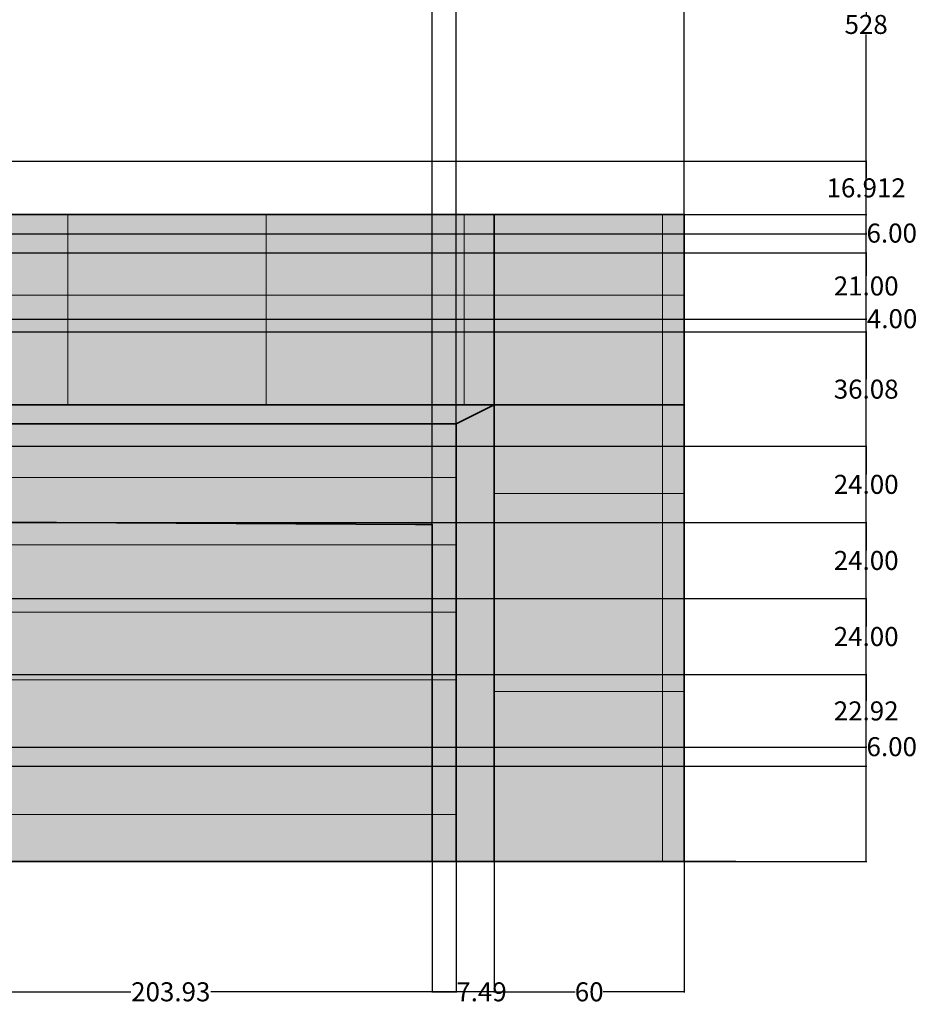
# Model space of a CAD drawing. Units: inches. Extents: x 148 to 1080, y 89 to 707.
# Tile 9 of 12: x 797 to 1080, y 89 to 399. Entities that reach past the tile are written whole.
import ezdxf

# ---------------------------------------------------------------- set-up
doc = ezdxf.new("R2010")
doc.units = ezdxf.units.IN
doc.header["$MEASUREMENT"] = 0
for name, color, linetype, lineweight in [('A-ANNO-DIMS', 2, 'Continuous', 18), ('A-ELEV', 7, 'Continuous', 35), ('A-ELEV-PATT', 8, 'Continuous', 13)]:
    doc.layers.add(name, color=color, linetype=linetype, lineweight=lineweight)
doc.styles.get("Standard").update_dxf_attribs({"font": 'arial.ttf'})
doc.dimstyles.get("Standard").update_dxf_attribs({"dimtxt": 6, "dimasz": 0.18, "dimexe": 0.18, "dimexo": 0.0625, "dimgap": 0.09, "dimtad": 0, "dimtih": 1, "dimtoh": 1, "dimdec": 0, "dimzin": 0, "dimdsep": 46, "dimlunit": 3, "dimtxsty": 'Standard', "dimcen": 0.09, "dimadec": 0, "dimazin": 0, "dimtfac": 1, "dimtdec": 0, "dimtofl": 0, "dimtmove": 0, "dimatfit": 3, "dimfxl": 1, "dimtolj": 1, "dimtzin": 0, "dimarcsym": 0})

# ---------------------------------------------------------------- blocks, each defined once
blk = doc.blocks.new('*D1')
at = {"layer": 'A-ANNO-DIMS', "color": 0, "lineweight": -2, "transparency": 16777216}
for p, q in [((215.02, 662.01), (215.02, 703.28)), ((215.2, 703.1), (604.32, 703.1)), ((1006.77, 703.1), (617.65, 703.1)), ((1006.95, 338.01), (1006.95, 703.28))]:
    blk.add_line(p, q, dxfattribs=at)
at = {"layer": 'A-ANNO-DIMS', "color": 0, "transparency": 16777216}
for points in [[(215.2, 703.13), (215.2, 703.07), (215.02, 703.1)], [(1006.77, 703.13), (1006.77, 703.07), (1006.95, 703.1)]]:
    blk.add_solid(points, dxfattribs=at)
at = {"layer": 'Defpoints', "color": 0, "transparency": 16777216}
for p in [(1006.95, 703.1), (215.02, 661.95), (1006.95, 337.95)]:
    blk.add_point(p, dxfattribs=at)
at = {"layer": 'A-ANNO-DIMS', "color": 0, "transparency": 16777216, "insert": (610.98, 703.1), "char_height": 6, "attachment_point": 5}
blk.add_mtext('\\A1;792', dxfattribs=at)
blk = doc.blocks.new('*D6')
at = {"layer": 'A-ANNO-DIMS', "color": 0, "lineweight": -2, "transparency": 16777216}
for p, q in [((743.02, 133.88), (743.02, 92.62)), ((946.95, 133.88), (946.95, 92.62)), ((743.2, 92.8), (832.39, 92.8)), ((946.77, 92.8), (857.58, 92.8))]:
    blk.add_line(p, q, dxfattribs=at)
at = {"layer": 'A-ANNO-DIMS', "color": 0, "transparency": 16777216}
for points in [[(743.2, 92.83), (743.2, 92.77), (743.02, 92.8)], [(946.77, 92.83), (946.77, 92.77), (946.95, 92.8)]]:
    blk.add_solid(points, dxfattribs=at)
at = {"layer": 'Defpoints', "color": 0, "transparency": 16777216}
for p in [(743.02, 133.95), (946.95, 133.95), (946.95, 92.8)]:
    blk.add_point(p, dxfattribs=at)
at = {"layer": 'A-ANNO-DIMS', "color": 0, "transparency": 16777216, "insert": (844.98, 92.8), "char_height": 6, "attachment_point": 5}
blk.add_mtext('\\A1;203.93', dxfattribs=at)
blk = doc.blocks.new('*D7')
at = {"layer": 'A-ANNO-DIMS', "color": 0, "lineweight": -2, "transparency": 16777216}
for p, q in [((946.95, 133.88), (946.95, 92.62)), ((1006.95, 133.88), (1006.95, 92.62)), ((947.13, 92.8), (972.56, 92.8)), ((1006.77, 92.8), (981.34, 92.8))]:
    blk.add_line(p, q, dxfattribs=at)
at = {"layer": 'A-ANNO-DIMS', "color": 0, "transparency": 16777216}
for points in [[(947.13, 92.83), (947.13, 92.77), (946.95, 92.8)], [(1006.77, 92.83), (1006.77, 92.77), (1006.95, 92.8)]]:
    blk.add_solid(points, dxfattribs=at)
at = {"layer": 'Defpoints', "color": 0, "transparency": 16777216}
for p in [(946.95, 133.95), (1006.95, 133.95), (1006.95, 92.8)]:
    blk.add_point(p, dxfattribs=at)
at = {"layer": 'A-ANNO-DIMS', "color": 0, "transparency": 16777216, "insert": (976.95, 92.8), "char_height": 6, "attachment_point": 5}
blk.add_mtext('\\A1;60', dxfattribs=at)
blk = doc.blocks.new('*D18')
at = {"layer": 'A-ANNO-DIMS', "color": 0, "lineweight": -2, "transparency": 16777216}
for p, q in [((635.08, 661.95), (1064.5, 661.95)), ((1064.32, 661.77), (1064.32, 401.1)), ((1064.32, 134.13), (1064.32, 394.79)), ((1007.01, 133.95), (1064.5, 133.95))]:
    blk.add_line(p, q, dxfattribs=at)
at = {"layer": 'A-ANNO-DIMS', "color": 0, "transparency": 16777216}
for points in [[(1064.29, 661.77), (1064.35, 661.77), (1064.32, 661.95)], [(1064.29, 134.13), (1064.35, 134.13), (1064.32, 133.95)]]:
    blk.add_solid(points, dxfattribs=at)
at = {"layer": 'Defpoints', "color": 0, "transparency": 16777216}
for p in [(635.02, 661.95), (1064.32, 661.95), (1006.95, 133.95)]:
    blk.add_point(p, dxfattribs=at)
at = {"layer": 'A-ANNO-DIMS', "color": 0, "transparency": 16777216, "insert": (1064.32, 397.95), "char_height": 6, "attachment_point": 5}
blk.add_mtext('\\A1;528', dxfattribs=at)
blk = doc.blocks.new('*D36')
at = {"layer": 'A-ANNO-DIMS', "color": 0, "lineweight": -2, "transparency": 16777216}
for p, q in [((765.95, 241.16), (765.95, 703.28)), ((766.13, 703.1), (844.01, 703.1)), ((934.77, 703.1), (856.89, 703.1)), ((934.95, 272.01), (934.95, 703.28))]:
    blk.add_line(p, q, dxfattribs=at)
at = {"layer": 'A-ANNO-DIMS', "color": 0, "transparency": 16777216}
for points in [[(766.13, 703.13), (766.13, 703.07), (765.95, 703.1)], [(934.77, 703.13), (934.77, 703.07), (934.95, 703.1)]]:
    blk.add_solid(points, dxfattribs=at)
at = {"layer": 'Defpoints', "color": 0, "transparency": 16777216}
for p in [(934.95, 703.1), (934.95, 271.95), (765.95, 241.1)]:
    blk.add_point(p, dxfattribs=at)
at = {"layer": 'A-ANNO-DIMS', "color": 0, "transparency": 16777216, "insert": (850.45, 703.1), "char_height": 6, "attachment_point": 5}
blk.add_mtext('\\A1;169', dxfattribs=at)
blk = doc.blocks.new('*D37')
at = {"layer": 'A-ANNO-DIMS', "color": 0, "lineweight": -2, "transparency": 16777216}
for p, q in [((765.95, 241.16), (765.95, 703.28)), ((766.13, 703.1), (836.75, 703.1)), ((927.28, 703.1), (856.66, 703.1)), ((927.46, 240.26), (927.46, 703.28))]:
    blk.add_line(p, q, dxfattribs=at)
at = {"layer": 'A-ANNO-DIMS', "color": 0, "transparency": 16777216}
for points in [[(766.13, 703.13), (766.13, 703.07), (765.95, 703.1)], [(927.28, 703.13), (927.28, 703.07), (927.46, 703.1)]]:
    blk.add_solid(points, dxfattribs=at)
at = {"layer": 'Defpoints', "color": 0, "transparency": 16777216}
for p in [(927.46, 703.1), (765.95, 241.1), (927.46, 240.2)]:
    blk.add_point(p, dxfattribs=at)
at = {"layer": 'A-ANNO-DIMS', "color": 0, "transparency": 16777216, "insert": (846.7, 703.1), "char_height": 6, "attachment_point": 5}
blk.add_mtext('\\A1;161.5', dxfattribs=at)
blk = doc.blocks.new('*D38')
at = {"layer": 'A-ANNO-DIMS', "color": 0, "lineweight": -2, "transparency": 16777216}
for p, q in [((934.89, 271.95), (160.42, 271.95)), ((160.6, 271.77), (160.6, 206.1)), ((160.6, 134.13), (160.6, 199.79)), ((934.89, 133.95), (160.42, 133.95))]:
    blk.add_line(p, q, dxfattribs=at)
at = {"layer": 'A-ANNO-DIMS', "color": 0, "transparency": 16777216}
for points in [[(160.57, 271.77), (160.63, 271.77), (160.6, 271.95)], [(160.57, 134.13), (160.63, 134.13), (160.6, 133.95)]]:
    blk.add_solid(points, dxfattribs=at)
at = {"layer": 'Defpoints', "color": 0, "transparency": 16777216}
for p in [(934.95, 271.95), (160.6, 133.95), (934.95, 133.95)]:
    blk.add_point(p, dxfattribs=at)
at = {"layer": 'A-ANNO-DIMS', "color": 0, "transparency": 16777216, "insert": (160.6, 202.95), "char_height": 6, "attachment_point": 5}
blk.add_mtext('\\A1;138', dxfattribs=at)
blk = doc.blocks.new('*D39')
at = {"layer": 'A-ANNO-DIMS', "color": 0, "lineweight": -2, "transparency": 16777216}
for p, q in [((946.89, 337.95), (160.42, 337.95)), ((160.6, 337.77), (160.6, 311.1)), ((160.6, 278.13), (160.6, 304.79)), ((946.89, 277.95), (160.42, 277.95))]:
    blk.add_line(p, q, dxfattribs=at)
at = {"layer": 'A-ANNO-DIMS', "color": 0, "transparency": 16777216}
for points in [[(160.57, 337.77), (160.63, 337.77), (160.6, 337.95)], [(160.57, 278.13), (160.63, 278.13), (160.6, 277.95)]]:
    blk.add_solid(points, dxfattribs=at)
at = {"layer": 'Defpoints', "color": 0, "transparency": 16777216}
for p in [(160.6, 337.95), (946.95, 337.95), (946.95, 277.95)]:
    blk.add_point(p, dxfattribs=at)
at = {"layer": 'A-ANNO-DIMS', "color": 0, "transparency": 16777216, "insert": (160.6, 307.95), "char_height": 6, "attachment_point": 5}
blk.add_mtext('\\A1;60', dxfattribs=at)
blk = doc.blocks.new('*D50')
at = {"layer": 'A-ANNO-DIMS', "color": 0, "lineweight": -2, "transparency": 16777216}
for p, q in [((727, 354.86), (1064.5, 354.86)), ((1064.32, 354.68), (1064.32, 349.56)), ((1064.32, 338.13), (1064.32, 343.25)), ((683.08, 337.95), (1064.5, 337.95))]:
    blk.add_line(p, q, dxfattribs=at)
at = {"layer": 'A-ANNO-DIMS', "color": 0, "transparency": 16777216}
for points in [[(1064.29, 354.68), (1064.35, 354.68), (1064.32, 354.86)], [(1064.29, 338.13), (1064.35, 338.13), (1064.32, 337.95)]]:
    blk.add_solid(points, dxfattribs=at)
at = {"layer": 'Defpoints', "color": 0, "transparency": 16777216}
for p in [(726.94, 354.86), (683.02, 337.95), (1064.32, 337.95)]:
    blk.add_point(p, dxfattribs=at)
at = {"layer": 'A-ANNO-DIMS', "color": 0, "transparency": 16777216, "insert": (1064.32, 346.4), "char_height": 6, "attachment_point": 5}
blk.add_mtext('\\A1;16.912', dxfattribs=at)
blk = doc.blocks.new('*D71')
at = {"layer": 'A-ANNO-DIMS', "color": 0, "lineweight": -2, "transparency": 16777216}
for p, q in [((389.08, 169.95), (1064.5, 169.95)), ((1064.32, 169.95), (1064.32, 170.13)), ((1064.32, 170.13), (1064.5, 170.13)), ((1064.32, 164.13), (1064.32, 169.77)), ((395.08, 163.95), (1064.5, 163.95))]:
    blk.add_line(p, q, dxfattribs=at)
at = {"layer": 'A-ANNO-DIMS', "color": 0, "transparency": 16777216}
for points in [[(1064.29, 169.77), (1064.35, 169.77), (1064.32, 169.95)], [(1064.29, 164.13), (1064.35, 164.13), (1064.32, 163.95)]]:
    blk.add_solid(points, dxfattribs=at)
at = {"layer": 'Defpoints', "color": 0, "transparency": 16777216}
for p in [(389.02, 169.95), (1064.32, 169.95), (395.02, 163.95)]:
    blk.add_point(p, dxfattribs=at)
at = {"layer": 'A-ANNO-DIMS', "color": 0, "transparency": 16777216, "insert": (1072.39, 170.13), "char_height": 6, "attachment_point": 5}
blk.add_mtext('\\A1;6.00', dxfattribs=at)
blk = doc.blocks.new('*D72')
at = {"layer": 'A-ANNO-DIMS', "color": 0, "lineweight": -2, "transparency": 16777216}
for p, q in [((389.08, 192.87), (1064.5, 192.87)), ((1064.32, 192.69), (1064.32, 184.56)), ((1064.32, 170.13), (1064.32, 178.26)), ((389.08, 169.95), (1064.5, 169.95))]:
    blk.add_line(p, q, dxfattribs=at)
at = {"layer": 'A-ANNO-DIMS', "color": 0, "transparency": 16777216}
for points in [[(1064.29, 192.69), (1064.35, 192.69), (1064.32, 192.87)], [(1064.29, 170.13), (1064.35, 170.13), (1064.32, 169.95)]]:
    blk.add_solid(points, dxfattribs=at)
at = {"layer": 'Defpoints', "color": 0, "transparency": 16777216}
for p in [(389.02, 192.87), (1064.32, 192.87), (389.02, 169.95)]:
    blk.add_point(p, dxfattribs=at)
at = {"layer": 'A-ANNO-DIMS', "color": 0, "transparency": 16777216, "insert": (1064.32, 181.41), "char_height": 6, "attachment_point": 5}
blk.add_mtext('\\A1;22.92', dxfattribs=at)
blk = doc.blocks.new('*D73')
at = {"layer": 'A-ANNO-DIMS', "color": 0, "lineweight": -2, "transparency": 16777216}
for p, q in [((389.08, 216.87), (1064.5, 216.87)), ((1064.32, 216.69), (1064.32, 208.02)), ((1064.32, 193.05), (1064.32, 201.72)), ((389.08, 192.87), (1064.5, 192.87))]:
    blk.add_line(p, q, dxfattribs=at)
at = {"layer": 'A-ANNO-DIMS', "color": 0, "transparency": 16777216}
for points in [[(1064.29, 216.69), (1064.35, 216.69), (1064.32, 216.87)], [(1064.29, 193.05), (1064.35, 193.05), (1064.32, 192.87)]]:
    blk.add_solid(points, dxfattribs=at)
at = {"layer": 'Defpoints', "color": 0, "transparency": 16777216}
for p in [(389.02, 216.87), (1064.32, 216.87), (389.02, 192.87)]:
    blk.add_point(p, dxfattribs=at)
at = {"layer": 'A-ANNO-DIMS', "color": 0, "transparency": 16777216, "insert": (1064.32, 204.87), "char_height": 6, "attachment_point": 5}
blk.add_mtext('\\A1;24.00', dxfattribs=at)
blk = doc.blocks.new('*D74')
at = {"layer": 'A-ANNO-DIMS', "color": 0, "lineweight": -2, "transparency": 16777216}
for p, q in [((389.08, 240.87), (1064.5, 240.87)), ((1064.32, 240.69), (1064.32, 232.02)), ((1064.32, 217.05), (1064.32, 225.72)), ((389.08, 216.87), (1064.5, 216.87))]:
    blk.add_line(p, q, dxfattribs=at)
at = {"layer": 'A-ANNO-DIMS', "color": 0, "transparency": 16777216}
for points in [[(1064.29, 240.69), (1064.35, 240.69), (1064.32, 240.87)], [(1064.29, 217.05), (1064.35, 217.05), (1064.32, 216.87)]]:
    blk.add_solid(points, dxfattribs=at)
at = {"layer": 'Defpoints', "color": 0, "transparency": 16777216}
for p in [(389.02, 240.87), (1064.32, 240.87), (389.02, 216.87)]:
    blk.add_point(p, dxfattribs=at)
at = {"layer": 'A-ANNO-DIMS', "color": 0, "transparency": 16777216, "insert": (1064.32, 228.87), "char_height": 6, "attachment_point": 5}
blk.add_mtext('\\A1;24.00', dxfattribs=at)
blk = doc.blocks.new('*D75')
at = {"layer": 'A-ANNO-DIMS', "color": 0, "lineweight": -2, "transparency": 16777216}
for p, q in [((389.08, 264.87), (1064.5, 264.87)), ((1064.32, 264.69), (1064.32, 256.02)), ((1064.32, 241.05), (1064.32, 249.72)), ((389.08, 240.87), (1064.5, 240.87))]:
    blk.add_line(p, q, dxfattribs=at)
at = {"layer": 'A-ANNO-DIMS', "color": 0, "transparency": 16777216}
for points in [[(1064.29, 264.69), (1064.35, 264.69), (1064.32, 264.87)], [(1064.29, 241.05), (1064.35, 241.05), (1064.32, 240.87)]]:
    blk.add_solid(points, dxfattribs=at)
at = {"layer": 'Defpoints', "color": 0, "transparency": 16777216}
for p in [(389.02, 264.87), (1064.32, 264.87), (389.02, 240.87)]:
    blk.add_point(p, dxfattribs=at)
at = {"layer": 'A-ANNO-DIMS', "color": 0, "transparency": 16777216, "insert": (1064.32, 252.87), "char_height": 6, "attachment_point": 5}
blk.add_mtext('\\A1;24.00', dxfattribs=at)
blk = doc.blocks.new('*D76')
at = {"layer": 'A-ANNO-DIMS', "color": 0, "lineweight": -2, "transparency": 16777216}
for p, q in [((389.08, 300.95), (1064.5, 300.95)), ((1064.32, 300.77), (1064.32, 286.06)), ((1064.32, 265.05), (1064.32, 279.75)), ((389.08, 264.87), (1064.5, 264.87))]:
    blk.add_line(p, q, dxfattribs=at)
at = {"layer": 'A-ANNO-DIMS', "color": 0, "transparency": 16777216}
for points in [[(1064.29, 300.77), (1064.35, 300.77), (1064.32, 300.95)], [(1064.29, 265.05), (1064.35, 265.05), (1064.32, 264.87)]]:
    blk.add_solid(points, dxfattribs=at)
at = {"layer": 'Defpoints', "color": 0, "transparency": 16777216}
for p in [(389.02, 300.95), (1064.32, 300.95), (389.02, 264.87)]:
    blk.add_point(p, dxfattribs=at)
at = {"layer": 'A-ANNO-DIMS', "color": 0, "transparency": 16777216, "insert": (1064.32, 282.91), "char_height": 6, "attachment_point": 5}
blk.add_mtext('\\A1;36.08', dxfattribs=at)
blk = doc.blocks.new('*D77')
at = {"layer": 'A-ANNO-DIMS', "color": 0, "lineweight": -2, "transparency": 16777216}
for p, q in [((389.08, 304.95), (1064.5, 304.95)), ((1064.32, 304.95), (1064.32, 305.13)), ((1064.32, 305.13), (1064.5, 305.13)), ((1064.32, 301.13), (1064.32, 304.77)), ((389.08, 300.95), (1064.5, 300.95))]:
    blk.add_line(p, q, dxfattribs=at)
at = {"layer": 'A-ANNO-DIMS', "color": 0, "transparency": 16777216}
for points in [[(1064.29, 304.77), (1064.35, 304.77), (1064.32, 304.95)], [(1064.29, 301.13), (1064.35, 301.13), (1064.32, 300.95)]]:
    blk.add_solid(points, dxfattribs=at)
at = {"layer": 'Defpoints', "color": 0, "transparency": 16777216}
for p in [(389.02, 304.95), (1064.32, 304.95), (389.02, 300.95)]:
    blk.add_point(p, dxfattribs=at)
at = {"layer": 'A-ANNO-DIMS', "color": 0, "transparency": 16777216, "insert": (1072.5, 305.13), "char_height": 6, "attachment_point": 5}
blk.add_mtext('\\A1;4.00', dxfattribs=at)
blk = doc.blocks.new('*D78')
at = {"layer": 'A-ANNO-DIMS', "color": 0, "lineweight": -2, "transparency": 16777216}
for p, q in [((389.08, 325.95), (1064.5, 325.95)), ((1064.32, 325.77), (1064.32, 318.6)), ((1064.32, 305.13), (1064.32, 312.29)), ((389.08, 304.95), (1064.5, 304.95))]:
    blk.add_line(p, q, dxfattribs=at)
at = {"layer": 'A-ANNO-DIMS', "color": 0, "transparency": 16777216}
for points in [[(1064.29, 325.77), (1064.35, 325.77), (1064.32, 325.95)], [(1064.29, 305.13), (1064.35, 305.13), (1064.32, 304.95)]]:
    blk.add_solid(points, dxfattribs=at)
at = {"layer": 'Defpoints', "color": 0, "transparency": 16777216}
for p in [(389.02, 325.95), (1064.32, 325.95), (389.02, 304.95)]:
    blk.add_point(p, dxfattribs=at)
at = {"layer": 'A-ANNO-DIMS', "color": 0, "transparency": 16777216, "insert": (1064.32, 315.45), "char_height": 6, "attachment_point": 5}
blk.add_mtext('\\A1;21.00', dxfattribs=at)
blk = doc.blocks.new('*D79')
at = {"layer": 'A-ANNO-DIMS', "color": 0, "lineweight": -2, "transparency": 16777216}
for p, q in [((395.08, 331.95), (1064.5, 331.95)), ((1064.32, 331.95), (1064.32, 332.13)), ((1064.32, 332.13), (1064.5, 332.13)), ((1064.32, 326.13), (1064.32, 331.77)), ((389.08, 325.95), (1064.5, 325.95))]:
    blk.add_line(p, q, dxfattribs=at)
at = {"layer": 'A-ANNO-DIMS', "color": 0, "transparency": 16777216}
for points in [[(1064.29, 331.77), (1064.35, 331.77), (1064.32, 331.95)], [(1064.29, 326.13), (1064.35, 326.13), (1064.32, 325.95)]]:
    blk.add_solid(points, dxfattribs=at)
at = {"layer": 'Defpoints', "color": 0, "transparency": 16777216}
for p in [(395.02, 331.95), (1064.32, 331.95), (389.02, 325.95)]:
    blk.add_point(p, dxfattribs=at)
at = {"layer": 'A-ANNO-DIMS', "color": 0, "transparency": 16777216, "insert": (1072.39, 332.13), "char_height": 6, "attachment_point": 5}
blk.add_mtext('\\A1;6.00', dxfattribs=at)
blk = doc.blocks.new('*D101')
at = {"layer": 'A-ANNO-DIMS', "color": 0, "lineweight": -2, "transparency": 16777216}
for p, q in [((927.46, 240.13), (927.46, 92.62)), ((934.95, 133.88), (934.95, 92.62)), ((927.64, 92.8), (934.77, 92.8)), ((934.95, 92.8), (935.13, 92.8))]:
    blk.add_line(p, q, dxfattribs=at)
at = {"layer": 'A-ANNO-DIMS', "color": 0, "transparency": 16777216}
for points in [[(927.64, 92.83), (927.64, 92.77), (927.46, 92.8)], [(934.77, 92.83), (934.77, 92.77), (934.95, 92.8)]]:
    blk.add_solid(points, dxfattribs=at)
at = {"layer": 'Defpoints', "color": 0, "transparency": 16777216}
for p in [(927.46, 240.2), (934.95, 133.95), (934.95, 92.8)]:
    blk.add_point(p, dxfattribs=at)
at = {"layer": 'A-ANNO-DIMS', "color": 0, "transparency": 16777216, "insert": (942.99, 92.8), "char_height": 6, "attachment_point": 5}
blk.add_mtext('\\A1;7.49', dxfattribs=at)

msp = doc.modelspace()

# ---------------------------------------------------------------- hatches: boundary and pattern name
at = {"layer": 'A-ELEV-PATT'}
h = msp.add_hatch(color=256, dxfattribs=at)
h.dxf.hatch_style = 1
h.paths.add_polyline_path([(527.0199, 272.3839), (395.0199, 271.2774), (395.0199, 163.9474), (275.0199, 163.9474), (275.0199, 270.2716), (251.0199, 270.0704), (251.0199, 133.9474), (527.0199, 133.9474)])
h.paths.add_polyline_path([(1006.9492, 337.9474), (946.9492, 337.9474), (946.9492, 277.9474), (1006.9492, 277.9474)])
h.paths.add_polyline_path([(1006.9492, 277.9474), (946.9492, 277.9474), (946.9492, 133.9474), (1006.9492, 133.9474)])
h.paths.add_polyline_path([(946.9492, 337.9474), (743.0199, 337.9474), (743.0199, 277.9474), (946.9492, 277.9474)])
h = msp.add_hatch(dxfattribs=at)
h.set_pattern_fill('ANSI37', color=256, scale=500, angle=135)
h.paths.add_polyline_path([(946.9492, 337.9474), (743.0199, 337.9474), (743.0199, 277.9474), (946.9492, 277.9474)])
h.paths.add_polyline_path([(1006.9492, 337.9474), (946.9492, 337.9474), (946.9492, 277.9474), (1006.9492, 277.9474)])
h.paths.add_polyline_path([(1006.9492, 277.9474), (946.9492, 277.9474), (946.9492, 133.9474), (1006.9492, 133.9474)])
h.paths.add_polyline_path([(719.0199, 337.9474), (683.0199, 337.9474), (683.0199, 133.9474), (719.0199, 133.9474)])
h.paths.add_polyline_path([(743.0199, 277.9474), (719.0199, 277.9474), (719.0199, 133.9474), (743.0199, 133.9474)])
h.paths.add_polyline_path([(743.0199, 337.9474), (734.0628, 337.9474), (719.0199, 326.3632), (719.0199, 277.9474), (743.0199, 277.9474)])
h.paths.add_polyline_path([(683.0199, 283.9474), (671.0199, 283.9474), (671.0199, 133.9474), (683.0199, 133.9474)])
h = msp.add_hatch(color=256, dxfattribs=at)
h.dxf.hatch_style = 1
h.paths.add_polyline_path([(946.9492, 277.9474), (743.0199, 277.9474), (743.0199, 271.9474), (934.9492, 271.9474)])
h.paths.add_polyline_path([(946.9492, 277.9474), (934.9492, 271.9474), (934.9492, 133.9474), (946.9492, 133.9474)])
h = msp.add_hatch(color=256, dxfattribs=at)
h.dxf.hatch_style = 1
h.paths.add_polyline_path([(934.9492, 271.9474), (743.0199, 271.9474), (743.0199, 133.9474), (776.713, 133.9474), (765.9474, 241.0996), (922.2028, 240.1776), (927.4587, 240.1966), (927.4587, 133.9474), (934.9492, 133.9474)])
h = msp.add_hatch(dxfattribs=at)
h.set_pattern_fill('ANSI31', color=256, scale=170, angle=135)
h.paths.add_polyline_path([(927.4587, 240.1966), (922.2028, 240.1776), (765.9474, 241.0996), (776.713, 133.9474), (927.4587, 133.9474)], flags=17)
h.paths.add_polyline_path([(934.9492, 271.9474), (743.0199, 271.9474), (743.0199, 133.9474), (776.713, 133.9474), (765.9474, 241.0996), (922.2028, 240.1776), (927.4587, 240.1966), (927.4587, 133.9474), (934.9492, 133.9474)])
h = msp.add_hatch(color=256, dxfattribs=at)
h.dxf.hatch_style = 1
h.paths.add_polyline_path([(927.4587, 240.1966), (922.2028, 240.1776), (765.9474, 241.0996), (776.713, 133.9474), (927.4587, 133.9474)])

# ---------------------------------------------------------------- linework, layer by layer
at = {"layer": 'A-ELEV'}
for p, q in [((527.0199, 337.9474), (1006.9492, 337.9474)), ((946.9492, 337.9474), (946.9492, 133.9474)), ((1006.9492, 337.9474), (1006.9492, 133.9474)), ((719.0199, 277.9474), (1006.9492, 277.9474)), ((946.9492, 277.9474), (934.9492, 271.9474)), ((743.0199, 271.9474), (934.9492, 271.9474)), ((934.9492, 271.9474), (934.9492, 133.9474)), ((765.9474, 241.0996), (922.2028, 240.1776)), ((922.2028, 240.1776), (927.4587, 240.1966)), ((927.4587, 240.1966), (927.4587, 133.9474)), ((201.7492, 133.9474), (1023.175, 133.9474))]:
    msp.add_line(p, q, dxfattribs=at)

# ---------------------------------------------------------------- dimensions: what is measured, and where the dimension line sits
at = {"layer": 'A-ANNO-DIMS'}
for base, p1, p2, override, picture, middle in [((1006.9492, 703.0974), (215.0199, 661.9474), (1006.9492, 337.9474), {"dimdec": 0, "dimlfac": 1, "dimrnd": 0, "dimzin": 0, "dimdsep": 46, "dimlunit": 2}, '*D1', (610.9845, 703.0974)), ((934.9492, 703.0974), (765.9474, 241.0996), (934.9492, 271.9474), {"dimdec": 0, "dimlfac": 1, "dimrnd": 0, "dimzin": 0, "dimdsep": 46, "dimlunit": 2}, '*D36', (850.4483, 703.0974)), ((927.4587, 703.0974), (765.9474, 241.0996), (927.4587, 240.1966), {"dimdec": 1, "dimlfac": 1, "dimrnd": 0, "dimzin": 0, "dimdsep": 46, "dimlunit": 2}, '*D37', (846.703, 703.0974)), ((934.9492, 92.7974), (927.4587, 240.1966), (934.9492, 133.9474), {"dimdec": 2, "dimlfac": 1, "dimrnd": 0, "dimzin": 0, "dimdsep": 46, "dimlunit": 2}, '*D101', (942.9934, 92.7974)), ((946.9492, 92.7974), (743.0199, 133.9474), (946.9492, 133.9474), {"dimdec": 2, "dimlfac": 1, "dimrnd": 0, "dimzin": 0, "dimdsep": 46, "dimlunit": 2}, '*D6', (844.9845, 92.7974)), ((1006.9492, 92.7974), (946.9492, 133.9474), (1006.9492, 133.9474), {"dimdec": 0, "dimlfac": 1, "dimrnd": 0, "dimzin": 0, "dimdsep": 46, "dimlunit": 2}, '*D7', (976.9492, 92.7974))]:
    dim = msp.add_linear_dim(base=base, p1=p1, p2=p2, dimstyle='Standard', override=override, dxfattribs=at)
    dim.commit()
    dim.dimension.update_dxf_attribs({"geometry": picture, "text_midpoint": middle})
for base, p1, p2, override, picture, middle in [((1064.325, 661.9474), (1006.9492, 133.9474), (635.0199, 661.9474), {"dimdec": 0, "dimlfac": 1, "dimrnd": 0, "dimzin": 0, "dimdsep": 46, "dimlunit": 2}, '*D18', (1064.325, 397.9474)), ((1064.325, 337.9474), (726.9419, 354.8591), (683.0199, 337.9474), {"dimdec": 3, "dimlfac": 1, "dimrnd": 0, "dimzin": 0, "dimdsep": 46, "dimlunit": 2}, '*D50', (1064.325, 346.4032)), ((160.5992, 337.9474), (946.9492, 277.9474), (946.9492, 337.9474), {"dimdec": 0, "dimlfac": 1, "dimrnd": 0, "dimzin": 0, "dimdsep": 46, "dimlunit": 2}, '*D39', (160.5992, 307.9474)), ((1064.325, 331.9474), (389.0199, 325.9474), (395.0199, 331.9474), {"dimdec": 2, "dimlfac": 1, "dimrnd": 0, "dimzin": 0, "dimdsep": 46, "dimlunit": 2}, '*D79', (1072.3937, 332.1274)), ((1064.325, 325.9474), (389.0199, 304.9474), (389.0199, 325.9474), {"dimdec": 2, "dimlfac": 1, "dimrnd": 0, "dimzin": 0, "dimdsep": 46, "dimlunit": 2}, '*D78', (1064.325, 315.4474)), ((1064.325, 304.9474), (389.0199, 300.9474), (389.0199, 304.9474), {"dimdec": 2, "dimlfac": 1, "dimrnd": 0, "dimzin": 0, "dimdsep": 46, "dimlunit": 2}, '*D77', (1072.4981, 305.1274)), ((1064.325, 300.9474), (389.0199, 264.8696), (389.0199, 300.9474), {"dimdec": 2, "dimlfac": 1, "dimrnd": 0, "dimzin": 0, "dimdsep": 46, "dimlunit": 2}, '*D76', (1064.325, 282.9085)), ((160.5992, 133.9474), (934.9492, 271.9474), (934.9492, 133.9474), {"dimdec": 0, "dimlfac": 1, "dimrnd": 0, "dimzin": 0, "dimdsep": 46, "dimlunit": 2}, '*D38', (160.5992, 202.9474)), ((1064.325, 264.8696), (389.0199, 240.8696), (389.0199, 264.8696), {"dimdec": 2, "dimlfac": 1, "dimrnd": 0, "dimzin": 0, "dimdsep": 46, "dimlunit": 2}, '*D75', (1064.325, 252.8696)), ((1064.325, 240.8696), (389.0199, 216.8696), (389.0199, 240.8696), {"dimdec": 2, "dimlfac": 1, "dimrnd": 0, "dimzin": 0, "dimdsep": 46, "dimlunit": 2}, '*D74', (1064.325, 228.8696)), ((1064.325, 216.8696), (389.0199, 192.8696), (389.0199, 216.8696), {"dimdec": 2, "dimlfac": 1, "dimrnd": 0, "dimzin": 0, "dimdsep": 46, "dimlunit": 2}, '*D73', (1064.325, 204.8696)), ((1064.325, 192.8696), (389.0199, 169.9474), (389.0199, 192.8696), {"dimdec": 2, "dimlfac": 1, "dimrnd": 0, "dimzin": 0, "dimdsep": 46, "dimlunit": 2}, '*D72', (1064.325, 181.4085)), ((1064.325, 169.9474), (395.0199, 163.9474), (389.0199, 169.9474), {"dimdec": 2, "dimlfac": 1, "dimrnd": 0, "dimzin": 0, "dimdsep": 46, "dimlunit": 2}, '*D71', (1072.3937, 170.1274))]:
    dim = msp.add_linear_dim(base=base, p1=p1, p2=p2, angle=90, dimstyle='Standard', override=override, dxfattribs=at)
    dim.commit()
    dim.dimension.update_dxf_attribs({"geometry": picture, "text_midpoint": middle})

doc.saveas('drawing.dxf')
